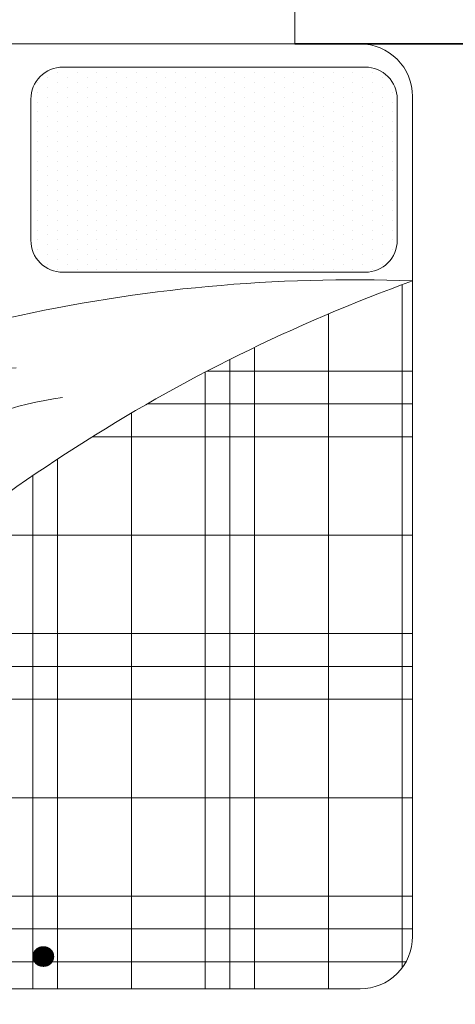
# Model space of a CAD drawing. Units: inches. Extents: x -269 to 4574, y -694 to 313.
# Tile 13 of 19: x 357 to 395, y -74 to 11. Entities that reach past the tile are written whole.
import ezdxf

# ---------------------------------------------------------------- set-up
doc = ezdxf.new("R2010")
doc.units = ezdxf.units.IN
doc.header["$MEASUREMENT"] = 0
for name, color, linetype, lineweight in [('A-FURN', 2, 'Continuous', 18), ('DIMENSION', 5, 'Continuous', 18), ('WALL', 1, 'Continuous', 35), ('WINDOWS', 2, 'Continuous', 18)]:
    doc.layers.add(name, color=color, linetype=linetype, lineweight=lineweight)
doc.dimstyles.get("Standard").update_dxf_attribs({"dimtxt": 10, "dimasz": 0.18, "dimexe": 0.18, "dimexo": 0.0625, "dimgap": 0.09, "dimtad": 0, "dimdec": 1, "dimzin": 0, "dimdsep": 46, "dimlunit": 3, "dimtxsty": 'Standard', "dimcen": 0.09, "dimclrt": 7, "dimadec": 0, "dimazin": 0, "dimtfac": 1, "dimtdec": 1, "dimtofl": 0, "dimtmove": 0, "dimatfit": 3, "dimfxl": 1, "dimtolj": 1, "dimtzin": 0, "dimarcsym": 0})

# ---------------------------------------------------------------- blocks, each defined once
blk = doc.blocks.new('*X12')
at = {"color": 0}
for p, q in [((273.75, 456.9375), (273.75, 456.9375)), ((273.9375, 457.03125), (273.9375, 457.03125)), ((274.125, 456.9375), (274.125, 456.9375)), ((274.3125, 457.03125), (274.3125, 457.03125)), ((274.5, 456.9375), (274.5, 456.9375)), ((274.6875, 457.03125), (274.6875, 457.03125)), ((274.875, 456.9375), (274.875, 456.9375)), ((275.0625, 457.03125), (275.0625, 457.03125)), ((275.25, 456.9375), (275.25, 456.9375)), ((275.4375, 457.03125), (275.4375, 457.03125)), ((275.625, 456.9375), (275.625, 456.9375)), ((275.8125, 457.03125), (275.8125, 457.03125)), ((276, 456.9375), (276, 456.9375)), ((276.1875, 457.03125), (276.1875, 457.03125)), ((276.375, 456.9375), (276.375, 456.9375)), ((276.5625, 457.03125), (276.5625, 457.03125)), ((276.75, 456.9375), (276.75, 456.9375)), ((276.9375, 457.03125), (276.9375, 457.03125)), ((277.125, 456.9375), (277.125, 456.9375)), ((277.3125, 457.03125), (277.3125, 457.03125)), ((277.5, 456.9375), (277.5, 456.9375)), ((277.6875, 457.03125), (277.6875, 457.03125)), ((277.875, 456.9375), (277.875, 456.9375)), ((278.0625, 457.03125), (278.0625, 457.03125)), ((278.25, 456.9375), (278.25, 456.9375)), ((278.4375, 457.03125), (278.4375, 457.03125)), ((278.625, 456.9375), (278.625, 456.9375)), ((278.8125, 457.03125), (278.8125, 457.03125)), ((279, 456.9375), (279, 456.9375)), ((279.1875, 457.03125), (279.1875, 457.03125)), ((279.375, 456.9375), (279.375, 456.9375)), ((279.5625, 457.03125), (279.5625, 457.03125)), ((279.75, 456.9375), (279.75, 456.9375)), ((273.375, 456.75), (273.375, 456.75)), ((273.5625, 456.84375), (273.5625, 456.84375)), ((273.75, 456.75), (273.75, 456.75)), ((273.9375, 456.84375), (273.9375, 456.84375)), ((274.125, 456.75), (274.125, 456.75)), ((274.3125, 456.84375), (274.3125, 456.84375)), ((274.5, 456.75), (274.5, 456.75)), ((274.6875, 456.84375), (274.6875, 456.84375)), ((274.875, 456.75), (274.875, 456.75)), ((275.0625, 456.84375), (275.0625, 456.84375)), ((275.25, 456.75), (275.25, 456.75)), ((275.4375, 456.84375), (275.4375, 456.84375)), ((275.625, 456.75), (275.625, 456.75)), ((275.8125, 456.84375), (275.8125, 456.84375)), ((276, 456.75), (276, 456.75)), ((276.1875, 456.84375), (276.1875, 456.84375)), ((276.375, 456.75), (276.375, 456.75)), ((276.5625, 456.84375), (276.5625, 456.84375)), ((276.75, 456.75), (276.75, 456.75)), ((276.9375, 456.84375), (276.9375, 456.84375)), ((277.125, 456.75), (277.125, 456.75)), ((277.3125, 456.84375), (277.3125, 456.84375)), ((277.5, 456.75), (277.5, 456.75)), ((277.6875, 456.84375), (277.6875, 456.84375)), ((277.875, 456.75), (277.875, 456.75)), ((278.0625, 456.84375), (278.0625, 456.84375)), ((278.25, 456.75), (278.25, 456.75)), ((278.4375, 456.84375), (278.4375, 456.84375)), ((278.625, 456.75), (278.625, 456.75)), ((278.8125, 456.84375), (278.8125, 456.84375)), ((279, 456.75), (279, 456.75)), ((279.1875, 456.84375), (279.1875, 456.84375)), ((279.375, 456.75), (279.375, 456.75)), ((279.5625, 456.84375), (279.5625, 456.84375)), ((279.75, 456.75), (279.75, 456.75)), ((279.9375, 456.84375), (279.9375, 456.84375)), ((280.125, 456.75), (280.125, 456.75)), ((273.375, 456.5625), (273.375, 456.5625)), ((273.5625, 456.65625), (273.5625, 456.65625)), ((273.75, 456.5625), (273.75, 456.5625)), ((273.9375, 456.65625), (273.9375, 456.65625)), ((274.125, 456.5625), (274.125, 456.5625)), ((274.3125, 456.65625), (274.3125, 456.65625)), ((274.5, 456.5625), (274.5, 456.5625)), ((274.6875, 456.65625), (274.6875, 456.65625)), ((274.875, 456.5625), (274.875, 456.5625)), ((275.0625, 456.65625), (275.0625, 456.65625)), ((275.25, 456.5625), (275.25, 456.5625)), ((275.4375, 456.65625), (275.4375, 456.65625)), ((275.625, 456.5625), (275.625, 456.5625)), ((275.8125, 456.65625), (275.8125, 456.65625)), ((276, 456.5625), (276, 456.5625)), ((276.1875, 456.65625), (276.1875, 456.65625)), ((276.375, 456.5625), (276.375, 456.5625)), ((276.5625, 456.65625), (276.5625, 456.65625)), ((276.75, 456.5625), (276.75, 456.5625)), ((276.9375, 456.65625), (276.9375, 456.65625)), ((277.125, 456.5625), (277.125, 456.5625)), ((277.3125, 456.65625), (277.3125, 456.65625)), ((277.5, 456.5625), (277.5, 456.5625)), ((277.6875, 456.65625), (277.6875, 456.65625)), ((277.875, 456.5625), (277.875, 456.5625)), ((278.0625, 456.65625), (278.0625, 456.65625)), ((278.25, 456.5625), (278.25, 456.5625)), ((278.4375, 456.65625), (278.4375, 456.65625)), ((278.625, 456.5625), (278.625, 456.5625)), ((278.8125, 456.65625), (278.8125, 456.65625)), ((279, 456.5625), (279, 456.5625)), ((279.1875, 456.65625), (279.1875, 456.65625)), ((279.375, 456.5625), (279.375, 456.5625)), ((279.5625, 456.65625), (279.5625, 456.65625)), ((279.75, 456.5625), (279.75, 456.5625)), ((279.9375, 456.65625), (279.9375, 456.65625)), ((280.125, 456.5625), (280.125, 456.5625)), ((273.375, 456.375), (273.375, 456.375)), ((273.5625, 456.46875), (273.5625, 456.46875)), ((273.75, 456.375), (273.75, 456.375)), ((273.9375, 456.46875), (273.9375, 456.46875)), ((274.125, 456.375), (274.125, 456.375)), ((274.3125, 456.46875), (274.3125, 456.46875)), ((274.5, 456.375), (274.5, 456.375)), ((274.6875, 456.46875), (274.6875, 456.46875)), ((274.875, 456.375), (274.875, 456.375)), ((275.0625, 456.46875), (275.0625, 456.46875)), ((275.25, 456.375), (275.25, 456.375)), ((275.4375, 456.46875), (275.4375, 456.46875)), ((275.625, 456.375), (275.625, 456.375)), ((275.8125, 456.46875), (275.8125, 456.46875)), ((276, 456.375), (276, 456.375)), ((276.1875, 456.46875), (276.1875, 456.46875)), ((276.375, 456.375), (276.375, 456.375)), ((276.5625, 456.46875), (276.5625, 456.46875)), ((276.75, 456.375), (276.75, 456.375)), ((276.9375, 456.46875), (276.9375, 456.46875)), ((277.125, 456.375), (277.125, 456.375)), ((277.3125, 456.46875), (277.3125, 456.46875)), ((277.5, 456.375), (277.5, 456.375)), ((277.6875, 456.46875), (277.6875, 456.46875)), ((277.875, 456.375), (277.875, 456.375)), ((278.0625, 456.46875), (278.0625, 456.46875)), ((278.25, 456.375), (278.25, 456.375)), ((278.4375, 456.46875), (278.4375, 456.46875)), ((278.625, 456.375), (278.625, 456.375)), ((278.8125, 456.46875), (278.8125, 456.46875)), ((279, 456.375), (279, 456.375)), ((279.1875, 456.46875), (279.1875, 456.46875)), ((279.375, 456.375), (279.375, 456.375)), ((279.5625, 456.46875), (279.5625, 456.46875)), ((279.75, 456.375), (279.75, 456.375)), ((279.9375, 456.46875), (279.9375, 456.46875)), ((280.125, 456.375), (280.125, 456.375)), ((273.375, 456.1875), (273.375, 456.1875)), ((273.5625, 456.28125), (273.5625, 456.28125)), ((273.75, 456.1875), (273.75, 456.1875)), ((273.9375, 456.28125), (273.9375, 456.28125)), ((274.125, 456.1875), (274.125, 456.1875)), ((274.3125, 456.28125), (274.3125, 456.28125)), ((274.5, 456.1875), (274.5, 456.1875)), ((274.6875, 456.28125), (274.6875, 456.28125)), ((274.875, 456.1875), (274.875, 456.1875)), ((275.0625, 456.28125), (275.0625, 456.28125)), ((275.25, 456.1875), (275.25, 456.1875)), ((275.4375, 456.28125), (275.4375, 456.28125)), ((275.625, 456.1875), (275.625, 456.1875)), ((275.8125, 456.28125), (275.8125, 456.28125)), ((276, 456.1875), (276, 456.1875)), ((276.1875, 456.28125), (276.1875, 456.28125)), ((276.375, 456.1875), (276.375, 456.1875)), ((276.5625, 456.28125), (276.5625, 456.28125)), ((276.75, 456.1875), (276.75, 456.1875)), ((276.9375, 456.28125), (276.9375, 456.28125)), ((277.125, 456.1875), (277.125, 456.1875)), ((277.3125, 456.28125), (277.3125, 456.28125)), ((277.5, 456.1875), (277.5, 456.1875)), ((277.6875, 456.28125), (277.6875, 456.28125)), ((277.875, 456.1875), (277.875, 456.1875)), ((278.0625, 456.28125), (278.0625, 456.28125)), ((278.25, 456.1875), (278.25, 456.1875)), ((278.4375, 456.28125), (278.4375, 456.28125)), ((278.625, 456.1875), (278.625, 456.1875)), ((278.8125, 456.28125), (278.8125, 456.28125)), ((279, 456.1875), (279, 456.1875)), ((279.1875, 456.28125), (279.1875, 456.28125)), ((279.375, 456.1875), (279.375, 456.1875)), ((279.5625, 456.28125), (279.5625, 456.28125)), ((279.75, 456.1875), (279.75, 456.1875)), ((279.9375, 456.28125), (279.9375, 456.28125)), ((280.125, 456.1875), (280.125, 456.1875)), ((273.375, 456), (273.375, 456)), ((273.5625, 456.09375), (273.5625, 456.09375)), ((273.75, 456), (273.75, 456)), ((273.9375, 456.09375), (273.9375, 456.09375)), ((274.125, 456), (274.125, 456)), ((274.3125, 456.09375), (274.3125, 456.09375)), ((274.5, 456), (274.5, 456)), ((274.6875, 456.09375), (274.6875, 456.09375)), ((274.875, 456), (274.875, 456)), ((275.0625, 456.09375), (275.0625, 456.09375)), ((275.25, 456), (275.25, 456)), ((275.4375, 456.09375), (275.4375, 456.09375)), ((275.625, 456), (275.625, 456)), ((275.8125, 456.09375), (275.8125, 456.09375)), ((276, 456), (276, 456)), ((276.1875, 456.09375), (276.1875, 456.09375)), ((276.375, 456), (276.375, 456)), ((276.5625, 456.09375), (276.5625, 456.09375)), ((276.75, 456), (276.75, 456)), ((276.9375, 456.09375), (276.9375, 456.09375)), ((277.125, 456), (277.125, 456)), ((277.3125, 456.09375), (277.3125, 456.09375)), ((277.5, 456), (277.5, 456)), ((277.6875, 456.09375), (277.6875, 456.09375)), ((277.875, 456), (277.875, 456)), ((278.0625, 456.09375), (278.0625, 456.09375)), ((278.25, 456), (278.25, 456)), ((278.4375, 456.09375), (278.4375, 456.09375)), ((278.625, 456), (278.625, 456)), ((278.8125, 456.09375), (278.8125, 456.09375)), ((279, 456), (279, 456)), ((279.1875, 456.09375), (279.1875, 456.09375)), ((279.375, 456), (279.375, 456)), ((279.5625, 456.09375), (279.5625, 456.09375)), ((279.75, 456), (279.75, 456)), ((279.9375, 456.09375), (279.9375, 456.09375)), ((280.125, 456), (280.125, 456)), ((273.375, 455.8125), (273.375, 455.8125)), ((273.5625, 455.90625), (273.5625, 455.90625)), ((273.75, 455.8125), (273.75, 455.8125)), ((273.9375, 455.90625), (273.9375, 455.90625)), ((274.125, 455.8125), (274.125, 455.8125)), ((274.3125, 455.90625), (274.3125, 455.90625)), ((274.5, 455.8125), (274.5, 455.8125)), ((274.6875, 455.90625), (274.6875, 455.90625)), ((274.875, 455.8125), (274.875, 455.8125)), ((275.0625, 455.90625), (275.0625, 455.90625)), ((275.25, 455.8125), (275.25, 455.8125)), ((275.4375, 455.90625), (275.4375, 455.90625)), ((275.625, 455.8125), (275.625, 455.8125)), ((275.8125, 455.90625), (275.8125, 455.90625)), ((276, 455.8125), (276, 455.8125)), ((276.1875, 455.90625), (276.1875, 455.90625)), ((276.375, 455.8125), (276.375, 455.8125)), ((276.5625, 455.90625), (276.5625, 455.90625)), ((276.75, 455.8125), (276.75, 455.8125)), ((276.9375, 455.90625), (276.9375, 455.90625)), ((277.125, 455.8125), (277.125, 455.8125)), ((277.3125, 455.90625), (277.3125, 455.90625)), ((277.5, 455.8125), (277.5, 455.8125)), ((277.6875, 455.90625), (277.6875, 455.90625)), ((277.875, 455.8125), (277.875, 455.8125)), ((278.0625, 455.90625), (278.0625, 455.90625)), ((278.25, 455.8125), (278.25, 455.8125)), ((278.4375, 455.90625), (278.4375, 455.90625)), ((278.625, 455.8125), (278.625, 455.8125)), ((278.8125, 455.90625), (278.8125, 455.90625)), ((279, 455.8125), (279, 455.8125)), ((279.1875, 455.90625), (279.1875, 455.90625)), ((279.375, 455.8125), (279.375, 455.8125)), ((279.5625, 455.90625), (279.5625, 455.90625)), ((279.75, 455.8125), (279.75, 455.8125)), ((279.9375, 455.90625), (279.9375, 455.90625)), ((280.125, 455.8125), (280.125, 455.8125)), ((273.375, 455.625), (273.375, 455.625)), ((273.5625, 455.71875), (273.5625, 455.71875)), ((273.75, 455.625), (273.75, 455.625)), ((273.9375, 455.71875), (273.9375, 455.71875)), ((274.125, 455.625), (274.125, 455.625)), ((274.3125, 455.71875), (274.3125, 455.71875)), ((274.5, 455.625), (274.5, 455.625)), ((274.6875, 455.71875), (274.6875, 455.71875)), ((274.875, 455.625), (274.875, 455.625)), ((275.0625, 455.71875), (275.0625, 455.71875)), ((275.25, 455.625), (275.25, 455.625)), ((275.4375, 455.71875), (275.4375, 455.71875)), ((275.625, 455.625), (275.625, 455.625)), ((275.8125, 455.71875), (275.8125, 455.71875)), ((276, 455.625), (276, 455.625)), ((276.1875, 455.71875), (276.1875, 455.71875)), ((276.375, 455.625), (276.375, 455.625)), ((276.5625, 455.71875), (276.5625, 455.71875)), ((276.75, 455.625), (276.75, 455.625)), ((276.9375, 455.71875), (276.9375, 455.71875)), ((277.125, 455.625), (277.125, 455.625)), ((277.3125, 455.71875), (277.3125, 455.71875)), ((277.5, 455.625), (277.5, 455.625)), ((277.6875, 455.71875), (277.6875, 455.71875)), ((277.875, 455.625), (277.875, 455.625)), ((278.0625, 455.71875), (278.0625, 455.71875)), ((278.25, 455.625), (278.25, 455.625)), ((278.4375, 455.71875), (278.4375, 455.71875)), ((278.625, 455.625), (278.625, 455.625)), ((278.8125, 455.71875), (278.8125, 455.71875)), ((279, 455.625), (279, 455.625)), ((279.1875, 455.71875), (279.1875, 455.71875)), ((279.375, 455.625), (279.375, 455.625)), ((279.5625, 455.71875), (279.5625, 455.71875)), ((279.75, 455.625), (279.75, 455.625)), ((279.9375, 455.71875), (279.9375, 455.71875)), ((280.125, 455.625), (280.125, 455.625)), ((273.375, 455.4375), (273.375, 455.4375)), ((273.5625, 455.53125), (273.5625, 455.53125)), ((273.75, 455.4375), (273.75, 455.4375)), ((273.9375, 455.53125), (273.9375, 455.53125)), ((274.125, 455.4375), (274.125, 455.4375)), ((274.3125, 455.53125), (274.3125, 455.53125)), ((274.5, 455.4375), (274.5, 455.4375)), ((274.6875, 455.53125), (274.6875, 455.53125)), ((274.875, 455.4375), (274.875, 455.4375)), ((275.0625, 455.53125), (275.0625, 455.53125)), ((275.25, 455.4375), (275.25, 455.4375)), ((275.4375, 455.53125), (275.4375, 455.53125)), ((275.625, 455.4375), (275.625, 455.4375)), ((275.8125, 455.53125), (275.8125, 455.53125)), ((276, 455.4375), (276, 455.4375)), ((276.1875, 455.53125), (276.1875, 455.53125)), ((276.375, 455.4375), (276.375, 455.4375)), ((276.5625, 455.53125), (276.5625, 455.53125)), ((276.75, 455.4375), (276.75, 455.4375)), ((276.9375, 455.53125), (276.9375, 455.53125)), ((277.125, 455.4375), (277.125, 455.4375)), ((277.3125, 455.53125), (277.3125, 455.53125)), ((277.5, 455.4375), (277.5, 455.4375)), ((277.6875, 455.53125), (277.6875, 455.53125)), ((277.875, 455.4375), (277.875, 455.4375)), ((278.0625, 455.53125), (278.0625, 455.53125)), ((278.25, 455.4375), (278.25, 455.4375)), ((278.4375, 455.53125), (278.4375, 455.53125)), ((278.625, 455.4375), (278.625, 455.4375)), ((278.8125, 455.53125), (278.8125, 455.53125)), ((279, 455.4375), (279, 455.4375)), ((279.1875, 455.53125), (279.1875, 455.53125)), ((279.375, 455.4375), (279.375, 455.4375)), ((279.5625, 455.53125), (279.5625, 455.53125)), ((279.75, 455.4375), (279.75, 455.4375)), ((279.9375, 455.53125), (279.9375, 455.53125)), ((280.125, 455.4375), (280.125, 455.4375)), ((273.375, 455.25), (273.375, 455.25)), ((273.5625, 455.34375), (273.5625, 455.34375)), ((273.75, 455.25), (273.75, 455.25)), ((273.9375, 455.34375), (273.9375, 455.34375)), ((274.125, 455.25), (274.125, 455.25)), ((274.3125, 455.34375), (274.3125, 455.34375)), ((274.5, 455.25), (274.5, 455.25)), ((274.6875, 455.34375), (274.6875, 455.34375)), ((274.875, 455.25), (274.875, 455.25)), ((275.0625, 455.34375), (275.0625, 455.34375)), ((275.25, 455.25), (275.25, 455.25)), ((275.4375, 455.34375), (275.4375, 455.34375)), ((275.625, 455.25), (275.625, 455.25)), ((275.8125, 455.34375), (275.8125, 455.34375)), ((276, 455.25), (276, 455.25)), ((276.1875, 455.34375), (276.1875, 455.34375)), ((276.375, 455.25), (276.375, 455.25)), ((276.5625, 455.34375), (276.5625, 455.34375)), ((276.75, 455.25), (276.75, 455.25)), ((276.9375, 455.34375), (276.9375, 455.34375)), ((277.125, 455.25), (277.125, 455.25)), ((277.3125, 455.34375), (277.3125, 455.34375)), ((277.5, 455.25), (277.5, 455.25)), ((277.6875, 455.34375), (277.6875, 455.34375)), ((277.875, 455.25), (277.875, 455.25)), ((278.0625, 455.34375), (278.0625, 455.34375)), ((278.25, 455.25), (278.25, 455.25)), ((278.4375, 455.34375), (278.4375, 455.34375)), ((278.625, 455.25), (278.625, 455.25)), ((278.8125, 455.34375), (278.8125, 455.34375)), ((279, 455.25), (279, 455.25)), ((279.1875, 455.34375), (279.1875, 455.34375)), ((279.375, 455.25), (279.375, 455.25)), ((279.5625, 455.34375), (279.5625, 455.34375)), ((279.75, 455.25), (279.75, 455.25)), ((279.9375, 455.34375), (279.9375, 455.34375)), ((280.125, 455.25), (280.125, 455.25)), ((273.375, 455.0625), (273.375, 455.0625)), ((273.5625, 455.15625), (273.5625, 455.15625)), ((273.75, 455.0625), (273.75, 455.0625)), ((273.9375, 455.15625), (273.9375, 455.15625)), ((274.125, 455.0625), (274.125, 455.0625)), ((274.3125, 455.15625), (274.3125, 455.15625)), ((274.5, 455.0625), (274.5, 455.0625)), ((274.6875, 455.15625), (274.6875, 455.15625)), ((274.875, 455.0625), (274.875, 455.0625)), ((275.0625, 455.15625), (275.0625, 455.15625)), ((275.25, 455.0625), (275.25, 455.0625)), ((275.4375, 455.15625), (275.4375, 455.15625)), ((275.625, 455.0625), (275.625, 455.0625)), ((275.8125, 455.15625), (275.8125, 455.15625)), ((276, 455.0625), (276, 455.0625)), ((276.1875, 455.15625), (276.1875, 455.15625)), ((276.375, 455.0625), (276.375, 455.0625)), ((276.5625, 455.15625), (276.5625, 455.15625)), ((276.75, 455.0625), (276.75, 455.0625)), ((276.9375, 455.15625), (276.9375, 455.15625)), ((277.125, 455.0625), (277.125, 455.0625)), ((277.3125, 455.15625), (277.3125, 455.15625)), ((277.5, 455.0625), (277.5, 455.0625)), ((277.6875, 455.15625), (277.6875, 455.15625)), ((277.875, 455.0625), (277.875, 455.0625)), ((278.0625, 455.15625), (278.0625, 455.15625)), ((278.25, 455.0625), (278.25, 455.0625)), ((278.4375, 455.15625), (278.4375, 455.15625)), ((278.625, 455.0625), (278.625, 455.0625)), ((278.8125, 455.15625), (278.8125, 455.15625)), ((279, 455.0625), (279, 455.0625)), ((279.1875, 455.15625), (279.1875, 455.15625)), ((279.375, 455.0625), (279.375, 455.0625)), ((279.5625, 455.15625), (279.5625, 455.15625)), ((279.75, 455.0625), (279.75, 455.0625)), ((279.9375, 455.15625), (279.9375, 455.15625)), ((280.125, 455.0625), (280.125, 455.0625)), ((273.375, 454.875), (273.375, 454.875)), ((273.5625, 454.96875), (273.5625, 454.96875)), ((273.75, 454.875), (273.75, 454.875)), ((273.9375, 454.96875), (273.9375, 454.96875)), ((274.125, 454.875), (274.125, 454.875)), ((274.3125, 454.96875), (274.3125, 454.96875)), ((274.5, 454.875), (274.5, 454.875)), ((274.6875, 454.96875), (274.6875, 454.96875)), ((274.875, 454.875), (274.875, 454.875)), ((275.0625, 454.96875), (275.0625, 454.96875)), ((275.25, 454.875), (275.25, 454.875)), ((275.4375, 454.96875), (275.4375, 454.96875)), ((275.625, 454.875), (275.625, 454.875)), ((275.8125, 454.96875), (275.8125, 454.96875)), ((276, 454.875), (276, 454.875)), ((276.1875, 454.96875), (276.1875, 454.96875)), ((276.375, 454.875), (276.375, 454.875)), ((276.5625, 454.96875), (276.5625, 454.96875)), ((276.75, 454.875), (276.75, 454.875)), ((276.9375, 454.96875), (276.9375, 454.96875)), ((277.125, 454.875), (277.125, 454.875)), ((277.3125, 454.96875), (277.3125, 454.96875)), ((277.5, 454.875), (277.5, 454.875)), ((277.6875, 454.96875), (277.6875, 454.96875)), ((277.875, 454.875), (277.875, 454.875)), ((278.0625, 454.96875), (278.0625, 454.96875)), ((278.25, 454.875), (278.25, 454.875)), ((278.4375, 454.96875), (278.4375, 454.96875)), ((278.625, 454.875), (278.625, 454.875)), ((278.8125, 454.96875), (278.8125, 454.96875)), ((279, 454.875), (279, 454.875)), ((279.1875, 454.96875), (279.1875, 454.96875)), ((279.375, 454.875), (279.375, 454.875)), ((279.5625, 454.96875), (279.5625, 454.96875)), ((279.75, 454.875), (279.75, 454.875)), ((279.9375, 454.96875), (279.9375, 454.96875)), ((280.125, 454.875), (280.125, 454.875)), ((273.375, 454.6875), (273.375, 454.6875)), ((273.5625, 454.78125), (273.5625, 454.78125)), ((273.75, 454.6875), (273.75, 454.6875)), ((273.9375, 454.78125), (273.9375, 454.78125)), ((274.125, 454.6875), (274.125, 454.6875)), ((274.3125, 454.78125), (274.3125, 454.78125)), ((274.5, 454.6875), (274.5, 454.6875)), ((274.6875, 454.78125), (274.6875, 454.78125)), ((274.875, 454.6875), (274.875, 454.6875)), ((275.0625, 454.78125), (275.0625, 454.78125)), ((275.25, 454.6875), (275.25, 454.6875)), ((275.4375, 454.78125), (275.4375, 454.78125)), ((275.625, 454.6875), (275.625, 454.6875)), ((275.8125, 454.78125), (275.8125, 454.78125)), ((276, 454.6875), (276, 454.6875)), ((276.1875, 454.78125), (276.1875, 454.78125)), ((276.375, 454.6875), (276.375, 454.6875)), ((276.5625, 454.78125), (276.5625, 454.78125)), ((276.75, 454.6875), (276.75, 454.6875)), ((276.9375, 454.78125), (276.9375, 454.78125)), ((277.125, 454.6875), (277.125, 454.6875)), ((277.3125, 454.78125), (277.3125, 454.78125)), ((277.5, 454.6875), (277.5, 454.6875)), ((277.6875, 454.78125), (277.6875, 454.78125)), ((277.875, 454.6875), (277.875, 454.6875)), ((278.0625, 454.78125), (278.0625, 454.78125)), ((278.25, 454.6875), (278.25, 454.6875)), ((278.4375, 454.78125), (278.4375, 454.78125)), ((278.625, 454.6875), (278.625, 454.6875)), ((278.8125, 454.78125), (278.8125, 454.78125)), ((279, 454.6875), (279, 454.6875)), ((279.1875, 454.78125), (279.1875, 454.78125)), ((279.375, 454.6875), (279.375, 454.6875)), ((279.5625, 454.78125), (279.5625, 454.78125)), ((279.75, 454.6875), (279.75, 454.6875)), ((279.9375, 454.78125), (279.9375, 454.78125)), ((280.125, 454.6875), (280.125, 454.6875)), ((273.375, 454.5), (273.375, 454.5)), ((273.5625, 454.59375), (273.5625, 454.59375)), ((273.75, 454.5), (273.75, 454.5)), ((273.9375, 454.59375), (273.9375, 454.59375)), ((274.125, 454.5), (274.125, 454.5)), ((274.3125, 454.59375), (274.3125, 454.59375)), ((274.5, 454.5), (274.5, 454.5)), ((274.6875, 454.59375), (274.6875, 454.59375)), ((274.875, 454.5), (274.875, 454.5)), ((275.0625, 454.59375), (275.0625, 454.59375)), ((275.25, 454.5), (275.25, 454.5)), ((275.4375, 454.59375), (275.4375, 454.59375)), ((275.625, 454.5), (275.625, 454.5)), ((275.8125, 454.59375), (275.8125, 454.59375)), ((276, 454.5), (276, 454.5)), ((276.1875, 454.59375), (276.1875, 454.59375)), ((276.375, 454.5), (276.375, 454.5)), ((276.5625, 454.59375), (276.5625, 454.59375)), ((276.75, 454.5), (276.75, 454.5)), ((276.9375, 454.59375), (276.9375, 454.59375)), ((277.125, 454.5), (277.125, 454.5)), ((277.3125, 454.59375), (277.3125, 454.59375)), ((277.5, 454.5), (277.5, 454.5)), ((277.6875, 454.59375), (277.6875, 454.59375)), ((277.875, 454.5), (277.875, 454.5)), ((278.0625, 454.59375), (278.0625, 454.59375)), ((278.25, 454.5), (278.25, 454.5)), ((278.4375, 454.59375), (278.4375, 454.59375)), ((278.625, 454.5), (278.625, 454.5)), ((278.8125, 454.59375), (278.8125, 454.59375)), ((279, 454.5), (279, 454.5)), ((279.1875, 454.59375), (279.1875, 454.59375)), ((279.375, 454.5), (279.375, 454.5)), ((279.5625, 454.59375), (279.5625, 454.59375)), ((279.75, 454.5), (279.75, 454.5)), ((279.9375, 454.59375), (279.9375, 454.59375)), ((280.125, 454.5), (280.125, 454.5)), ((273.375, 454.3125), (273.375, 454.3125)), ((273.5625, 454.40625), (273.5625, 454.40625)), ((273.75, 454.3125), (273.75, 454.3125)), ((273.9375, 454.40625), (273.9375, 454.40625)), ((274.125, 454.3125), (274.125, 454.3125)), ((274.3125, 454.40625), (274.3125, 454.40625)), ((274.5, 454.3125), (274.5, 454.3125)), ((274.6875, 454.40625), (274.6875, 454.40625)), ((274.875, 454.3125), (274.875, 454.3125)), ((275.0625, 454.40625), (275.0625, 454.40625)), ((275.25, 454.3125), (275.25, 454.3125)), ((275.4375, 454.40625), (275.4375, 454.40625)), ((275.625, 454.3125), (275.625, 454.3125)), ((275.8125, 454.40625), (275.8125, 454.40625)), ((276, 454.3125), (276, 454.3125)), ((276.1875, 454.40625), (276.1875, 454.40625)), ((276.375, 454.3125), (276.375, 454.3125)), ((276.5625, 454.40625), (276.5625, 454.40625)), ((276.75, 454.3125), (276.75, 454.3125)), ((276.9375, 454.40625), (276.9375, 454.40625)), ((277.125, 454.3125), (277.125, 454.3125)), ((277.3125, 454.40625), (277.3125, 454.40625)), ((277.5, 454.3125), (277.5, 454.3125)), ((277.6875, 454.40625), (277.6875, 454.40625)), ((277.875, 454.3125), (277.875, 454.3125)), ((278.0625, 454.40625), (278.0625, 454.40625)), ((278.25, 454.3125), (278.25, 454.3125)), ((278.4375, 454.40625), (278.4375, 454.40625)), ((278.625, 454.3125), (278.625, 454.3125)), ((278.8125, 454.40625), (278.8125, 454.40625)), ((279, 454.3125), (279, 454.3125)), ((279.1875, 454.40625), (279.1875, 454.40625)), ((279.375, 454.3125), (279.375, 454.3125)), ((279.5625, 454.40625), (279.5625, 454.40625)), ((279.75, 454.3125), (279.75, 454.3125)), ((279.9375, 454.40625), (279.9375, 454.40625)), ((280.125, 454.3125), (280.125, 454.3125)), ((273.375, 454.125), (273.375, 454.125)), ((273.5625, 454.21875), (273.5625, 454.21875)), ((273.75, 454.125), (273.75, 454.125)), ((273.9375, 454.21875), (273.9375, 454.21875)), ((274.125, 454.125), (274.125, 454.125)), ((274.3125, 454.21875), (274.3125, 454.21875)), ((274.5, 454.125), (274.5, 454.125)), ((274.6875, 454.21875), (274.6875, 454.21875)), ((274.875, 454.125), (274.875, 454.125)), ((275.0625, 454.21875), (275.0625, 454.21875)), ((275.25, 454.125), (275.25, 454.125)), ((275.4375, 454.21875), (275.4375, 454.21875)), ((275.625, 454.125), (275.625, 454.125)), ((275.8125, 454.21875), (275.8125, 454.21875)), ((276, 454.125), (276, 454.125)), ((276.1875, 454.21875), (276.1875, 454.21875)), ((276.375, 454.125), (276.375, 454.125)), ((276.5625, 454.21875), (276.5625, 454.21875)), ((276.75, 454.125), (276.75, 454.125)), ((276.9375, 454.21875), (276.9375, 454.21875)), ((277.125, 454.125), (277.125, 454.125)), ((277.3125, 454.21875), (277.3125, 454.21875)), ((277.5, 454.125), (277.5, 454.125)), ((277.6875, 454.21875), (277.6875, 454.21875)), ((277.875, 454.125), (277.875, 454.125)), ((278.0625, 454.21875), (278.0625, 454.21875)), ((278.25, 454.125), (278.25, 454.125)), ((278.4375, 454.21875), (278.4375, 454.21875)), ((278.625, 454.125), (278.625, 454.125)), ((278.8125, 454.21875), (278.8125, 454.21875)), ((279, 454.125), (279, 454.125)), ((279.1875, 454.21875), (279.1875, 454.21875)), ((279.375, 454.125), (279.375, 454.125)), ((279.5625, 454.21875), (279.5625, 454.21875)), ((279.75, 454.125), (279.75, 454.125)), ((279.9375, 454.21875), (279.9375, 454.21875)), ((280.125, 454.125), (280.125, 454.125)), ((273.375, 453.9375), (273.375, 453.9375)), ((273.5625, 454.03125), (273.5625, 454.03125)), ((273.75, 453.9375), (273.75, 453.9375)), ((273.9375, 454.03125), (273.9375, 454.03125)), ((274.125, 453.9375), (274.125, 453.9375)), ((274.3125, 454.03125), (274.3125, 454.03125)), ((274.5, 453.9375), (274.5, 453.9375)), ((274.6875, 454.03125), (274.6875, 454.03125)), ((274.875, 453.9375), (274.875, 453.9375)), ((275.0625, 454.03125), (275.0625, 454.03125)), ((275.25, 453.9375), (275.25, 453.9375)), ((275.4375, 454.03125), (275.4375, 454.03125)), ((275.625, 453.9375), (275.625, 453.9375)), ((275.8125, 454.03125), (275.8125, 454.03125)), ((276, 453.9375), (276, 453.9375)), ((276.1875, 454.03125), (276.1875, 454.03125)), ((276.375, 453.9375), (276.375, 453.9375)), ((276.5625, 454.03125), (276.5625, 454.03125)), ((276.75, 453.9375), (276.75, 453.9375)), ((276.9375, 454.03125), (276.9375, 454.03125)), ((277.125, 453.9375), (277.125, 453.9375)), ((277.3125, 454.03125), (277.3125, 454.03125)), ((277.5, 453.9375), (277.5, 453.9375)), ((277.6875, 454.03125), (277.6875, 454.03125)), ((277.875, 453.9375), (277.875, 453.9375)), ((278.0625, 454.03125), (278.0625, 454.03125)), ((278.25, 453.9375), (278.25, 453.9375)), ((278.4375, 454.03125), (278.4375, 454.03125)), ((278.625, 453.9375), (278.625, 453.9375)), ((278.8125, 454.03125), (278.8125, 454.03125)), ((279, 453.9375), (279, 453.9375)), ((279.1875, 454.03125), (279.1875, 454.03125)), ((279.375, 453.9375), (279.375, 453.9375)), ((279.5625, 454.03125), (279.5625, 454.03125)), ((279.75, 453.9375), (279.75, 453.9375)), ((279.9375, 454.03125), (279.9375, 454.03125)), ((280.125, 453.9375), (280.125, 453.9375)), ((273.375, 453.75), (273.375, 453.75)), ((273.5625, 453.84375), (273.5625, 453.84375)), ((273.75, 453.75), (273.75, 453.75)), ((273.9375, 453.84375), (273.9375, 453.84375)), ((274.125, 453.75), (274.125, 453.75)), ((274.3125, 453.84375), (274.3125, 453.84375)), ((274.5, 453.75), (274.5, 453.75)), ((274.6875, 453.84375), (274.6875, 453.84375)), ((274.875, 453.75), (274.875, 453.75)), ((275.0625, 453.84375), (275.0625, 453.84375)), ((275.25, 453.75), (275.25, 453.75)), ((275.4375, 453.84375), (275.4375, 453.84375)), ((275.625, 453.75), (275.625, 453.75)), ((275.8125, 453.84375), (275.8125, 453.84375)), ((276, 453.75), (276, 453.75)), ((276.1875, 453.84375), (276.1875, 453.84375)), ((276.375, 453.75), (276.375, 453.75)), ((276.5625, 453.84375), (276.5625, 453.84375)), ((276.75, 453.75), (276.75, 453.75)), ((276.9375, 453.84375), (276.9375, 453.84375)), ((277.125, 453.75), (277.125, 453.75)), ((277.3125, 453.84375), (277.3125, 453.84375)), ((277.5, 453.75), (277.5, 453.75)), ((277.6875, 453.84375), (277.6875, 453.84375)), ((277.875, 453.75), (277.875, 453.75)), ((278.0625, 453.84375), (278.0625, 453.84375)), ((278.25, 453.75), (278.25, 453.75)), ((278.4375, 453.84375), (278.4375, 453.84375)), ((278.625, 453.75), (278.625, 453.75)), ((278.8125, 453.84375), (278.8125, 453.84375)), ((279, 453.75), (279, 453.75)), ((279.1875, 453.84375), (279.1875, 453.84375)), ((279.375, 453.75), (279.375, 453.75)), ((279.5625, 453.84375), (279.5625, 453.84375)), ((279.75, 453.75), (279.75, 453.75)), ((279.9375, 453.84375), (279.9375, 453.84375)), ((280.125, 453.75), (280.125, 453.75)), ((273.375, 453.5625), (273.375, 453.5625)), ((273.5625, 453.65625), (273.5625, 453.65625)), ((273.75, 453.5625), (273.75, 453.5625)), ((273.9375, 453.65625), (273.9375, 453.65625)), ((274.125, 453.5625), (274.125, 453.5625)), ((274.3125, 453.65625), (274.3125, 453.65625)), ((274.5, 453.5625), (274.5, 453.5625)), ((274.6875, 453.65625), (274.6875, 453.65625)), ((274.875, 453.5625), (274.875, 453.5625)), ((275.0625, 453.65625), (275.0625, 453.65625)), ((275.25, 453.5625), (275.25, 453.5625)), ((275.4375, 453.65625), (275.4375, 453.65625)), ((275.625, 453.5625), (275.625, 453.5625)), ((275.8125, 453.65625), (275.8125, 453.65625)), ((276, 453.5625), (276, 453.5625)), ((276.1875, 453.65625), (276.1875, 453.65625)), ((276.375, 453.5625), (276.375, 453.5625)), ((276.5625, 453.65625), (276.5625, 453.65625)), ((276.75, 453.5625), (276.75, 453.5625)), ((276.9375, 453.65625), (276.9375, 453.65625)), ((277.125, 453.5625), (277.125, 453.5625)), ((277.3125, 453.65625), (277.3125, 453.65625)), ((277.5, 453.5625), (277.5, 453.5625)), ((277.6875, 453.65625), (277.6875, 453.65625)), ((277.875, 453.5625), (277.875, 453.5625)), ((278.0625, 453.65625), (278.0625, 453.65625)), ((278.25, 453.5625), (278.25, 453.5625)), ((278.4375, 453.65625), (278.4375, 453.65625)), ((278.625, 453.5625), (278.625, 453.5625)), ((278.8125, 453.65625), (278.8125, 453.65625)), ((279, 453.5625), (279, 453.5625)), ((279.1875, 453.65625), (279.1875, 453.65625)), ((279.375, 453.5625), (279.375, 453.5625)), ((279.5625, 453.65625), (279.5625, 453.65625)), ((279.75, 453.5625), (279.75, 453.5625)), ((279.9375, 453.65625), (279.9375, 453.65625)), ((280.125, 453.5625), (280.125, 453.5625)), ((273.375, 453.375), (273.375, 453.375)), ((273.5625, 453.46875), (273.5625, 453.46875)), ((273.75, 453.375), (273.75, 453.375)), ((273.9375, 453.46875), (273.9375, 453.46875)), ((274.125, 453.375), (274.125, 453.375)), ((274.3125, 453.46875), (274.3125, 453.46875)), ((274.5, 453.375), (274.5, 453.375)), ((274.6875, 453.46875), (274.6875, 453.46875)), ((274.875, 453.375), (274.875, 453.375)), ((275.0625, 453.46875), (275.0625, 453.46875)), ((275.25, 453.375), (275.25, 453.375)), ((275.4375, 453.46875), (275.4375, 453.46875)), ((275.625, 453.375), (275.625, 453.375)), ((275.8125, 453.46875), (275.8125, 453.46875)), ((276, 453.375), (276, 453.375)), ((276.1875, 453.46875), (276.1875, 453.46875)), ((276.375, 453.375), (276.375, 453.375)), ((276.5625, 453.46875), (276.5625, 453.46875)), ((276.75, 453.375), (276.75, 453.375)), ((276.9375, 453.46875), (276.9375, 453.46875)), ((277.125, 453.375), (277.125, 453.375)), ((277.3125, 453.46875), (277.3125, 453.46875)), ((277.5, 453.375), (277.5, 453.375)), ((277.6875, 453.46875), (277.6875, 453.46875)), ((277.875, 453.375), (277.875, 453.375)), ((278.0625, 453.46875), (278.0625, 453.46875)), ((278.25, 453.375), (278.25, 453.375)), ((278.4375, 453.46875), (278.4375, 453.46875)), ((278.625, 453.375), (278.625, 453.375)), ((278.8125, 453.46875), (278.8125, 453.46875)), ((279, 453.375), (279, 453.375)), ((279.1875, 453.46875), (279.1875, 453.46875)), ((279.375, 453.375), (279.375, 453.375)), ((279.5625, 453.46875), (279.5625, 453.46875)), ((279.75, 453.375), (279.75, 453.375)), ((279.9375, 453.46875), (279.9375, 453.46875)), ((273.5625, 453.28125), (273.5625, 453.28125)), ((273.75, 453.1875), (273.75, 453.1875)), ((273.9375, 453.28125), (273.9375, 453.28125)), ((274.125, 453.1875), (274.125, 453.1875)), ((274.3125, 453.28125), (274.3125, 453.28125)), ((274.5, 453.1875), (274.5, 453.1875)), ((274.6875, 453.28125), (274.6875, 453.28125)), ((274.875, 453.1875), (274.875, 453.1875)), ((275.0625, 453.28125), (275.0625, 453.28125)), ((275.25, 453.1875), (275.25, 453.1875)), ((275.4375, 453.28125), (275.4375, 453.28125)), ((275.625, 453.1875), (275.625, 453.1875)), ((275.8125, 453.28125), (275.8125, 453.28125)), ((276, 453.1875), (276, 453.1875)), ((276.1875, 453.28125), (276.1875, 453.28125)), ((276.375, 453.1875), (276.375, 453.1875)), ((276.5625, 453.28125), (276.5625, 453.28125)), ((276.75, 453.1875), (276.75, 453.1875)), ((276.9375, 453.28125), (276.9375, 453.28125)), ((277.125, 453.1875), (277.125, 453.1875)), ((277.3125, 453.28125), (277.3125, 453.28125)), ((277.5, 453.1875), (277.5, 453.1875)), ((277.6875, 453.28125), (277.6875, 453.28125)), ((277.875, 453.1875), (277.875, 453.1875)), ((278.0625, 453.28125), (278.0625, 453.28125)), ((278.25, 453.1875), (278.25, 453.1875)), ((278.4375, 453.28125), (278.4375, 453.28125)), ((278.625, 453.1875), (278.625, 453.1875)), ((278.8125, 453.28125), (278.8125, 453.28125)), ((279, 453.1875), (279, 453.1875)), ((279.1875, 453.28125), (279.1875, 453.28125)), ((279.375, 453.1875), (279.375, 453.1875)), ((279.5625, 453.28125), (279.5625, 453.28125)), ((279.75, 453.1875), (279.75, 453.1875)), ((279.9375, 453.28125), (279.9375, 453.28125))]:
    blk.add_line(p, q, dxfattribs=at)
blk = doc.blocks.new('GLAZ-48IN')
blk.add_line((4.5, 0), (4.5, 48))
blk.add_lwpolyline([(0, 48), (9, 48), (9, 0), (0, 0)], close=True)
blk = doc.blocks.new('*X10')
at = {"color": 0}
for p, q in [((276.598, 451.25), (280.51, 451.25)), ((275.455, 450.625), (280.51, 450.625)), ((274.411, 450), (280.51, 450)), ((265.51, 448.125), (267.634, 448.125)), ((271.723, 448.125), (280.51, 448.125)), ((265.51, 446.25), (268.465, 446.25)), ((269.519, 446.25), (280.51, 446.25)), ((265.51, 445.625), (268.531, 445.625)), ((268.866, 445.625), (280.51, 445.625)), ((265.51, 445), (280.51, 445)), ((265.51, 443.125), (280.51, 443.125)), ((265.51, 441.25), (280.51, 441.25)), ((265.51, 440.625), (280.51, 440.625)), ((265.634, 440), (280.386, 440))]:
    blk.add_line(p, q, dxfattribs=at)
blk = doc.blocks.new('*X11')
at = {"color": 0}
for p, q in [((280.312, 439.886), (280.312, 452.896)), ((278.906, 439.482), (278.906, 452.338)), ((277.5, 439.482), (277.5, 451.702)), ((277.031, 439.482), (277.031, 451.471)), ((276.562, 439.482), (276.562, 451.231)), ((275.156, 439.482), (275.156, 450.451)), ((273.75, 439.482), (273.75, 449.576)), ((265.781, 439.797), (265.781, 449.511)), ((266.25, 439.517), (266.25, 449.296)), ((273.281, 439.482), (273.281, 449.261)), ((272.812, 439.482), (272.812, 448.934)), ((267.656, 439.482), (267.656, 448.095)), ((271.406, 439.482), (271.406, 447.876)), ((270, 439.482), (270, 446.689)), ((269.531, 439.482), (269.531, 446.262)), ((269.062, 439.482), (269.062, 445.817))]:
    blk.add_line(p, q, dxfattribs=at)
blk = doc.blocks.new('BED-DOUBLE-COVER')
for centre, radius, start, end in [((63.323, -75.959), 137.598, 87.86419, 117.40011), ((118.648, -76.93), 147.291, 109.92605, 135.39771), ((36.861, 17.247), 36.854, 94.44362, 133.27876), ((41.517, 23.741), 27.874, 97.21567, 147.66565), ((-5.916, 27.396), 19.714, 357.37917, 72.5379)]:
    blk.add_arc(centre, radius, start, end)
at = {"xscale": 4.5633847399786, "yscale": 4.5633847399786, "zscale": 4.5633847399786}
for name in ['*X11', '*X10']:
    blk.add_blockref(name, (-1211.623, -2005.527), dxfattribs=at)
blk = doc.blocks.new('*D49')
at = {"layer": 'Defpoints', "color": 0, "lineweight": 0, "transparency": 16777216}
for p in [(344.278, -221.793), (354.546, -221.793), (344.278, -290.244)]:
    blk.add_point(p, dxfattribs=at)
at = {"layer": 'DIMENSION', "color": 0, "lineweight": -2, "transparency": 16777216}
for p, q in [((354.546, -221.793), (354.546, -221.613)), ((344.34, -221.793), (354.726, -221.793)), ((354.546, -290.064), (354.546, -221.973)), ((344.34, -290.244), (354.726, -290.244))]:
    blk.add_line(p, q, dxfattribs=at)
at = {"layer": 'DIMENSION', "color": 0, "lineweight": 0, "transparency": 16777216}
for points in [[(354.516, -221.973), (354.576, -221.973), (354.546, -221.793)], [(354.516, -290.064), (354.576, -290.064), (354.546, -290.244)]]:
    blk.add_solid(points, dxfattribs=at)
at = {"layer": 'DIMENSION', "color": 7, "transparency": 16777216, "insert": (354.546, -133.666), "char_height": 10, "attachment_point": 5, "rotation": 90}
blk.add_mtext('\\A1;COVER 5\'-8 1/2" TYP.', dxfattribs=at)

msp = doc.modelspace()

# ---------------------------------------------------------------- linework, layer by layer
at = {"layer": 'A-FURN'}
for points in [[(386.299, -72.873), (326.975, -72.873, -0.414214), (322.412, -68.309), (322.412, 4.705, -0.414214), (326.975, 9.268), (386.299, 9.268, -0.414214), (390.862, 4.705), (390.862, -68.309, -0.414214)], [(386.754, -10.579), (360.472, -10.579, -0.414214), (357.695, -7.802), (357.695, 4.469, -0.414214), (360.472, 7.246), (386.754, 7.246, -0.414214), (389.531, 4.469), (389.531, -7.802, -0.414214)]]:
    msp.add_lwpolyline(points, format="xyb", close=True, dxfattribs=at)
at = {"layer": 'WALL'}
msp.add_line((380.637, 9.268), (442.137, 9.268), dxfattribs=at)

# ---------------------------------------------------------------- block references
at = {"layer": 'A-FURN', "xscale": 4.5633847399786, "yscale": 4.5633847399786, "zscale": 4.5633847399786}
msp.add_blockref('*X12', (-889.211, -2078.4), dxfattribs=at)
at = {"layer": 'A-FURN'}
msp.add_blockref('BED-DOUBLE-COVER', (322.412, -72.873), dxfattribs=at)
at = {"layer": 'WINDOWS', "extrusion": (0, 0, -1), "zscale": -1, "rotation": 269.9999999999999}
msp.add_blockref('GLAZ-48IN', (-380.637, 18.268), dxfattribs=at)

# ---------------------------------------------------------------- dimensions: what is measured, and where the dimension line sits
at = {"layer": 'DIMENSION'}
dim = msp.add_linear_dim(base=(354.546, -221.793), p1=(344.278, -290.244), p2=(344.278, -221.793), angle=90, text='COVER <> TYP.', dimstyle='Standard', override={"dimdec": 1, "dimlfac": 1, "dimrnd": 0, "dimzin": 1, "dimdsep": 46, "dimlunit": 4, "dimfrac": 2}, dxfattribs=at)
dim.commit()
dim.dimension.update_dxf_attribs({"geometry": '*D49', "text_midpoint": (354.546, -133.666)})

doc.saveas('drawing.dxf')
